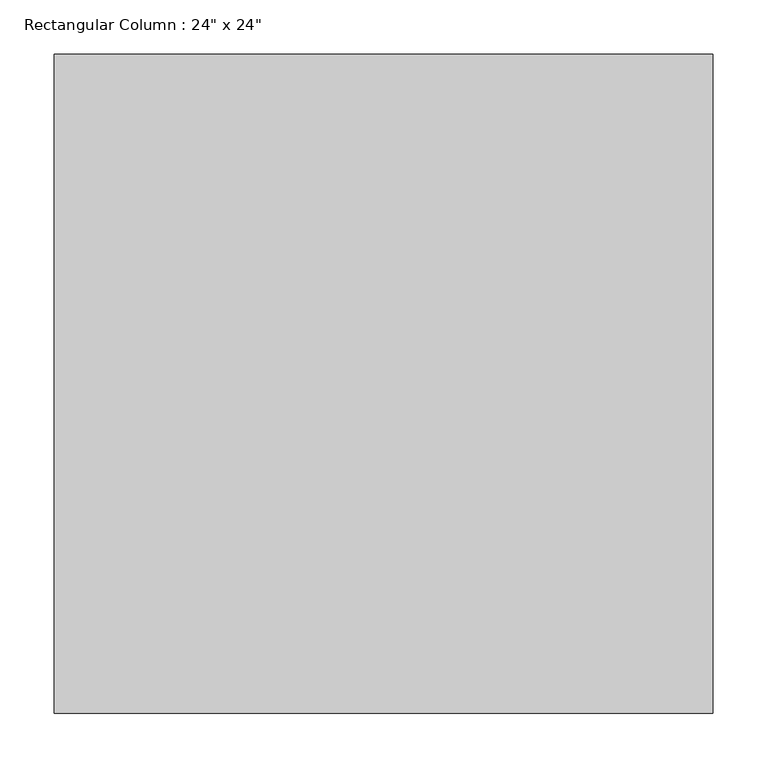
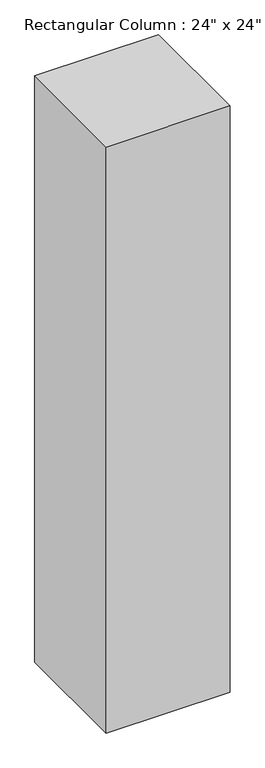
"""IFC4 building model written with IfcOpenShell, lengths in millimetres: column geometry."""

from ifc_helpers import new_model, si_unit, origin, origin_with_axes, place, context, project, spatial, polyline, outline, extrude, source, transform, mapped, element, save


def column_c091e905(model_context):
    return source(origin(), model_context, "Body", "SweptSolid", [
        extrude(outline(polyline([(304.8, 304.8), (304.8, -304.8), (-304.8, -304.8), (-304.8, 304.8), (304.8, 304.8)])), origin_with_axes(), (0.0, 0.0, 1.0), 3048.0),
    ])


if __name__ == "__main__":
    model = new_model("IFC4")
    model_context = context("Model", 3, world=origin())
    ifc_project = project(units=[si_unit("LENGTHUNIT", "METRE", prefix="MILLI")], contexts=[model_context])
    site = spatial("IfcSite", under=ifc_project)
    building = spatial("IfcBuilding", under=site)
    placement = place(None, origin())
    column_shape = column_c091e905(model_context)
    element("IfcColumn", 1, ObjectType="Rectangular Column : 24\" x 24\"", at=placement, inside=building, context=model_context, shape_type="MappedRepresentation", body=[
        mapped(column_shape, transform((0.0, 0.0, 0.0), x_axis=(1.0, 0.0, 0.0), y_axis=(0.0, 1.0, 0.0), z_axis=(0.0, 0.0, 1.0))),
    ])
    save(model, "model.ifc")

# Revit data of these elements
# Type "Rectangular Column : 24\" x 24\""
#   Assembly Code = "B1010200"
#   Depth = 2' - 0"
#   Offset Base = 0' - 0"
#   Offset Top = 0' - 0"
#   Width = 2' - 0"
#   Material = none
